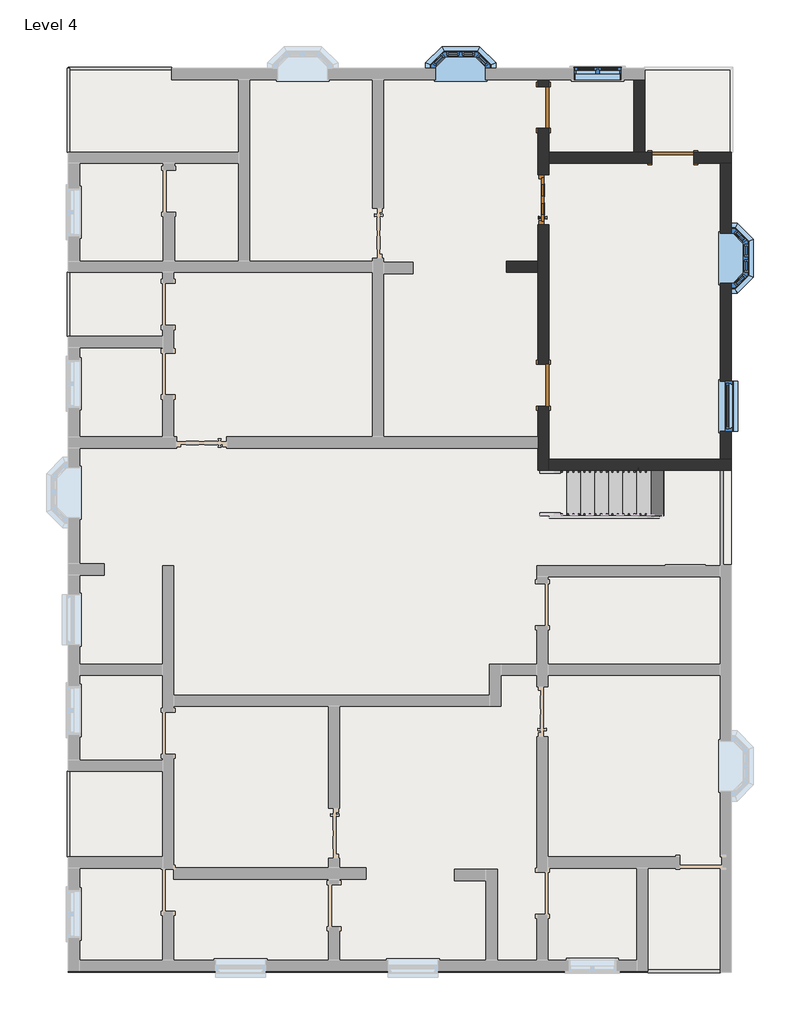
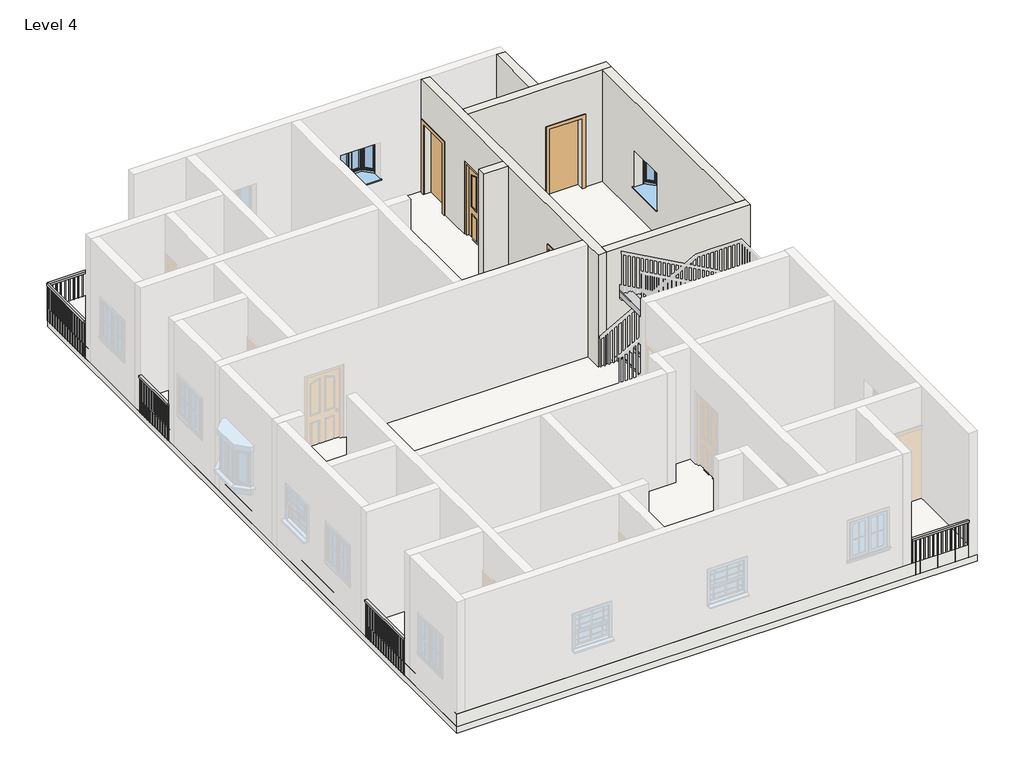
# One storey, part 2 of 4: 6 walls, 5 railings, 4 doors, 4 windows, 1 roof, 1 slab, 1 stair flight.
"""IFC4 building model written with IfcOpenShell, lengths in millimetres."""

from ifc_helpers import new_model, si_unit, frame, origin, place, context, project, spatial, polyline, outline, extrude, faceted_brep, transform, mapped, element, save
from components import doors_extsgl_12_910x2110mm_9a09825e, door_53b1b562, stair_flight_b1286695, window_910x910mm_67ef725a, window_c29befe5, windows_sash_w_bars_1_910x910mm_b688f793

model = new_model("IFC4")

# Units and contexts
model_context = context("Model", 3, world=origin())
ifc_project = project(units=[si_unit("LENGTHUNIT", "METRE", prefix="MILLI")], contexts=[model_context])

# Site, building, storey
site = spatial("IfcSite", under=ifc_project)
building = spatial("IfcBuilding", under=site)
storey = spatial("IfcBuildingStorey", under=building, Name="Level 4", Elevation=9144.0)

# Doors
placement = place(None, origin())
doors_extsgl_12_910x2110mm_shape = doors_extsgl_12_910x2110mm_9a09825e(model_context)
element("IfcDoor", 1, ObjectType="Doors_ExtSgl_12 : 910x2110mm", at=placement, inside=storey, context=model_context, shape_type="MappedRepresentation", body=[
    mapped(doors_extsgl_12_910x2110mm_shape, transform((1600.6941283, 5934.0547293, 9144.0), x_axis=(0.0, 1.0, 0.0), y_axis=(-1.0, 0.0, 0.0), z_axis=(0.0, 0.0, 1.0))),
])
door_shape = door_53b1b562(model_context)
element("IfcDoor", 2, ObjectType="Single-Flush : 30\" x 80\"", at=placement, inside=storey, context=model_context, shape_type="MappedRepresentation", body=[
    mapped(door_shape, transform((1600.6941283, 2555.8547293, 9144.0), x_axis=(0.0, 1.0, 0.0), y_axis=(-1.0, 0.0, 0.0), z_axis=(0.0, 0.0, 1.0))),
])
element("IfcDoor", 3, ObjectType="Single-Flush : 30\" x 80\"", at=placement, inside=storey, context=model_context, shape_type="MappedRepresentation", body=[
    mapped(door_shape, transform((1600.6941283, 7610.4547293, 9144.0), x_axis=(0.0, 1.0, 0.0), y_axis=(-1.0, 0.0, 0.0), z_axis=(0.0, 0.0, 1.0))),
])
element("IfcDoor", 4, ObjectType="Single-Flush : 30\" x 80\"", at=placement, inside=storey, context=model_context, shape_type="MappedRepresentation", body=[
    mapped(door_shape, transform((3962.8941283, 6696.0547293, 9144.0), x_axis=(-1.0, 0.0, 0.0), y_axis=(0.0, -1.0, 0.0), z_axis=(0.0, 0.0, 1.0))),
])

# Railings
element("IfcRailing", 5, ObjectType="Handrail - Rectangular", at=placement, inside=storey, context=model_context, shape_type="SweptSolid", body=[
    extrude(outline(polyline([(-7073.4058717, 4609.0339901), (-7022.6058717, 4609.0339901), (-7022.6058717, 3444.8547293), (-7073.4058717, 3444.8547293), (-7073.4058717, 4609.0339901)])), frame((0.0, 0.0, 10007.6), z_axis=(0.0, 0.0, 1.0), x_axis=(1.0, 0.0, 0.0)), (0.0, 0.0, 1.0), 50.8),
    extrude(outline(polyline([(-7057.5308717, 3500.9589901), (-7038.4808717, 3500.9589901), (-7038.4808717, 3481.9089901), (-7057.5308717, 3481.9089901), (-7057.5308717, 3500.9589901)])), frame((0.0, 0.0, 9144.0), z_axis=(0.0, 0.0, 1.0), x_axis=(1.0, 0.0, 0.0)), (0.0, 0.0, 1.0), 863.6),
    extrude(outline(polyline([(-7057.5308717, 3602.5589901), (-7038.4808717, 3602.5589901), (-7038.4808717, 3583.5089901), (-7057.5308717, 3583.5089901), (-7057.5308717, 3602.5589901)])), frame((0.0, 0.0, 9144.0), z_axis=(0.0, 0.0, 1.0), x_axis=(1.0, 0.0, 0.0)), (0.0, 0.0, 1.0), 863.6),
    extrude(outline(polyline([(-7057.5308717, 3704.1589901), (-7038.4808717, 3704.1589901), (-7038.4808717, 3685.1089901), (-7057.5308717, 3685.1089901), (-7057.5308717, 3704.1589901)])), frame((0.0, 0.0, 9144.0), z_axis=(0.0, 0.0, 1.0), x_axis=(1.0, 0.0, 0.0)), (0.0, 0.0, 1.0), 863.6),
    extrude(outline(polyline([(-7057.5308717, 3805.7589901), (-7038.4808717, 3805.7589901), (-7038.4808717, 3786.7089901), (-7057.5308717, 3786.7089901), (-7057.5308717, 3805.7589901)])), frame((0.0, 0.0, 9144.0), z_axis=(0.0, 0.0, 1.0), x_axis=(1.0, 0.0, 0.0)), (0.0, 0.0, 1.0), 863.6),
    extrude(outline(polyline([(-7057.5308717, 3907.3589901), (-7038.4808717, 3907.3589901), (-7038.4808717, 3888.3089901), (-7057.5308717, 3888.3089901), (-7057.5308717, 3907.3589901)])), frame((0.0, 0.0, 9144.0), z_axis=(0.0, 0.0, 1.0), x_axis=(1.0, 0.0, 0.0)), (0.0, 0.0, 1.0), 863.6),
    extrude(outline(polyline([(-7057.5308717, 4008.9589901), (-7038.4808717, 4008.9589901), (-7038.4808717, 3989.9089901), (-7057.5308717, 3989.9089901), (-7057.5308717, 4008.9589901)])), frame((0.0, 0.0, 9144.0), z_axis=(0.0, 0.0, 1.0), x_axis=(1.0, 0.0, 0.0)), (0.0, 0.0, 1.0), 863.6),
    extrude(outline(polyline([(-7057.5308717, 4110.5589901), (-7038.4808717, 4110.5589901), (-7038.4808717, 4091.5089901), (-7057.5308717, 4091.5089901), (-7057.5308717, 4110.5589901)])), frame((0.0, 0.0, 9144.0), z_axis=(0.0, 0.0, 1.0), x_axis=(1.0, 0.0, 0.0)), (0.0, 0.0, 1.0), 863.6),
    extrude(outline(polyline([(-7057.5308717, 4212.1589901), (-7038.4808717, 4212.1589901), (-7038.4808717, 4193.1089901), (-7057.5308717, 4193.1089901), (-7057.5308717, 4212.1589901)])), frame((0.0, 0.0, 9144.0), z_axis=(0.0, 0.0, 1.0), x_axis=(1.0, 0.0, 0.0)), (0.0, 0.0, 1.0), 863.6),
    extrude(outline(polyline([(-7057.5308717, 4313.7589901), (-7038.4808717, 4313.7589901), (-7038.4808717, 4294.7089901), (-7057.5308717, 4294.7089901), (-7057.5308717, 4313.7589901)])), frame((0.0, 0.0, 9144.0), z_axis=(0.0, 0.0, 1.0), x_axis=(1.0, 0.0, 0.0)), (0.0, 0.0, 1.0), 863.6),
    extrude(outline(polyline([(-7057.5308717, 4415.3589901), (-7038.4808717, 4415.3589901), (-7038.4808717, 4396.3089901), (-7057.5308717, 4396.3089901), (-7057.5308717, 4415.3589901)])), frame((0.0, 0.0, 9144.0), z_axis=(0.0, 0.0, 1.0), x_axis=(1.0, 0.0, 0.0)), (0.0, 0.0, 1.0), 863.6),
    extrude(outline(polyline([(-7057.5308717, 4516.9589901), (-7038.4808717, 4516.9589901), (-7038.4808717, 4497.9089901), (-7057.5308717, 4497.9089901), (-7057.5308717, 4516.9589901)])), frame((0.0, 0.0, 9144.0), z_axis=(0.0, 0.0, 1.0), x_axis=(1.0, 0.0, 0.0)), (0.0, 0.0, 1.0), 863.6),
    extrude(outline(polyline([(-7057.5308717, 3463.9047293), (-7038.4808717, 3463.9047293), (-7038.4808717, 3444.8547293), (-7057.5308717, 3444.8547293), (-7057.5308717, 3463.9047293)])), frame((0.0, 0.0, 9144.0), z_axis=(0.0, 0.0, 1.0), x_axis=(1.0, 0.0, 0.0)), (0.0, 0.0, 1.0), 863.6),
    extrude(outline(polyline([(-7057.5308717, 4609.0339901), (-7038.4808717, 4609.0339901), (-7038.4808717, 4589.9839901), (-7057.5308717, 4589.9839901), (-7057.5308717, 4609.0339901)])), frame((0.0, 0.0, 9144.0), z_axis=(0.0, 0.0, 1.0), x_axis=(1.0, 0.0, 0.0)), (0.0, 0.0, 1.0), 863.6),
])
element("IfcRailing", 6, ObjectType="Handrail - Rectangular", at=placement, inside=storey, context=model_context, shape_type="SweptSolid", body=[
    extrude(outline(polyline([(-7073.4058717, -4474.6886333), (-7022.6058717, -4474.6886333), (-7022.6058717, -6029.3452707), (-7073.4058717, -6029.3452707), (-7073.4058717, -4474.6886333)])), frame((0.0, 0.0, 10007.6), z_axis=(0.0, 0.0, 1.0), x_axis=(1.0, 0.0, 0.0)), (0.0, 0.0, 1.0), 50.8),
    extrude(outline(polyline([(-7057.5308717, -5989.1636333), (-7038.4808717, -5989.1636333), (-7038.4808717, -6008.2136333), (-7057.5308717, -6008.2136333), (-7057.5308717, -5989.1636333)])), frame((0.0, 0.0, 9144.0), z_axis=(0.0, 0.0, 1.0), x_axis=(1.0, 0.0, 0.0)), (0.0, 0.0, 1.0), 863.6),
    extrude(outline(polyline([(-7057.5308717, -5887.5636333), (-7038.4808717, -5887.5636333), (-7038.4808717, -5906.6136333), (-7057.5308717, -5906.6136333), (-7057.5308717, -5887.5636333)])), frame((0.0, 0.0, 9144.0), z_axis=(0.0, 0.0, 1.0), x_axis=(1.0, 0.0, 0.0)), (0.0, 0.0, 1.0), 863.6),
    extrude(outline(polyline([(-7057.5308717, -5785.9636333), (-7038.4808717, -5785.9636333), (-7038.4808717, -5805.0136333), (-7057.5308717, -5805.0136333), (-7057.5308717, -5785.9636333)])), frame((0.0, 0.0, 9144.0), z_axis=(0.0, 0.0, 1.0), x_axis=(1.0, 0.0, 0.0)), (0.0, 0.0, 1.0), 863.6),
    extrude(outline(polyline([(-7057.5308717, -5684.3636333), (-7038.4808717, -5684.3636333), (-7038.4808717, -5703.4136333), (-7057.5308717, -5703.4136333), (-7057.5308717, -5684.3636333)])), frame((0.0, 0.0, 9144.0), z_axis=(0.0, 0.0, 1.0), x_axis=(1.0, 0.0, 0.0)), (0.0, 0.0, 1.0), 863.6),
    extrude(outline(polyline([(-7057.5308717, -5582.7636333), (-7038.4808717, -5582.7636333), (-7038.4808717, -5601.8136333), (-7057.5308717, -5601.8136333), (-7057.5308717, -5582.7636333)])), frame((0.0, 0.0, 9144.0), z_axis=(0.0, 0.0, 1.0), x_axis=(1.0, 0.0, 0.0)), (0.0, 0.0, 1.0), 863.6),
    extrude(outline(polyline([(-7057.5308717, -5481.1636333), (-7038.4808717, -5481.1636333), (-7038.4808717, -5500.2136333), (-7057.5308717, -5500.2136333), (-7057.5308717, -5481.1636333)])), frame((0.0, 0.0, 9144.0), z_axis=(0.0, 0.0, 1.0), x_axis=(1.0, 0.0, 0.0)), (0.0, 0.0, 1.0), 863.6),
    extrude(outline(polyline([(-7057.5308717, -5379.5636333), (-7038.4808717, -5379.5636333), (-7038.4808717, -5398.6136333), (-7057.5308717, -5398.6136333), (-7057.5308717, -5379.5636333)])), frame((0.0, 0.0, 9144.0), z_axis=(0.0, 0.0, 1.0), x_axis=(1.0, 0.0, 0.0)), (0.0, 0.0, 1.0), 863.6),
    extrude(outline(polyline([(-7057.5308717, -5277.9636333), (-7038.4808717, -5277.9636333), (-7038.4808717, -5297.0136333), (-7057.5308717, -5297.0136333), (-7057.5308717, -5277.9636333)])), frame((0.0, 0.0, 9144.0), z_axis=(0.0, 0.0, 1.0), x_axis=(1.0, 0.0, 0.0)), (0.0, 0.0, 1.0), 863.6),
    extrude(outline(polyline([(-7057.5308717, -5176.3636333), (-7038.4808717, -5176.3636333), (-7038.4808717, -5195.4136333), (-7057.5308717, -5195.4136333), (-7057.5308717, -5176.3636333)])), frame((0.0, 0.0, 9144.0), z_axis=(0.0, 0.0, 1.0), x_axis=(1.0, 0.0, 0.0)), (0.0, 0.0, 1.0), 863.6),
    extrude(outline(polyline([(-7057.5308717, -5074.7636333), (-7038.4808717, -5074.7636333), (-7038.4808717, -5093.8136333), (-7057.5308717, -5093.8136333), (-7057.5308717, -5074.7636333)])), frame((0.0, 0.0, 9144.0), z_axis=(0.0, 0.0, 1.0), x_axis=(1.0, 0.0, 0.0)), (0.0, 0.0, 1.0), 863.6),
    extrude(outline(polyline([(-7057.5308717, -4973.1636333), (-7038.4808717, -4973.1636333), (-7038.4808717, -4992.2136333), (-7057.5308717, -4992.2136333), (-7057.5308717, -4973.1636333)])), frame((0.0, 0.0, 9144.0), z_axis=(0.0, 0.0, 1.0), x_axis=(1.0, 0.0, 0.0)), (0.0, 0.0, 1.0), 863.6),
    extrude(outline(polyline([(-7057.5308717, -4871.5636333), (-7038.4808717, -4871.5636333), (-7038.4808717, -4890.6136333), (-7057.5308717, -4890.6136333), (-7057.5308717, -4871.5636333)])), frame((0.0, 0.0, 9144.0), z_axis=(0.0, 0.0, 1.0), x_axis=(1.0, 0.0, 0.0)), (0.0, 0.0, 1.0), 863.6),
    extrude(outline(polyline([(-7057.5308717, -4769.9636333), (-7038.4808717, -4769.9636333), (-7038.4808717, -4789.0136333), (-7057.5308717, -4789.0136333), (-7057.5308717, -4769.9636333)])), frame((0.0, 0.0, 9144.0), z_axis=(0.0, 0.0, 1.0), x_axis=(1.0, 0.0, 0.0)), (0.0, 0.0, 1.0), 863.6),
    extrude(outline(polyline([(-7057.5308717, -4668.3636333), (-7038.4808717, -4668.3636333), (-7038.4808717, -4687.4136333), (-7057.5308717, -4687.4136333), (-7057.5308717, -4668.3636333)])), frame((0.0, 0.0, 9144.0), z_axis=(0.0, 0.0, 1.0), x_axis=(1.0, 0.0, 0.0)), (0.0, 0.0, 1.0), 863.6),
    extrude(outline(polyline([(-7057.5308717, -4566.7636333), (-7038.4808717, -4566.7636333), (-7038.4808717, -4585.8136333), (-7057.5308717, -4585.8136333), (-7057.5308717, -4566.7636333)])), frame((0.0, 0.0, 9144.0), z_axis=(0.0, 0.0, 1.0), x_axis=(1.0, 0.0, 0.0)), (0.0, 0.0, 1.0), 863.6),
    extrude(outline(polyline([(-7057.5308717, -6010.2952707), (-7038.4808717, -6010.2952707), (-7038.4808717, -6029.3452707), (-7057.5308717, -6029.3452707), (-7057.5308717, -6010.2952707)])), frame((0.0, 0.0, 9144.0), z_axis=(0.0, 0.0, 1.0), x_axis=(1.0, 0.0, 0.0)), (0.0, 0.0, 1.0), 863.6),
    extrude(outline(polyline([(-7057.5308717, -4474.6886333), (-7038.4808717, -4474.6886333), (-7038.4808717, -4493.7386333), (-7057.5308717, -4493.7386333), (-7057.5308717, -4474.6886333)])), frame((0.0, 0.0, 9144.0), z_axis=(0.0, 0.0, 1.0), x_axis=(1.0, 0.0, 0.0)), (0.0, 0.0, 1.0), 863.6),
])
element("IfcRailing", 7, ObjectType="Handrail - Rectangular", at=placement, inside=storey, context=model_context, shape_type="SweptSolid", body=[
    extrude(outline(polyline([(3505.6941283, -8137.5452707), (3505.6941283, -8086.7452707), (4826.4941283, -8086.7452707), (4826.4941283, -8137.5452707), (3505.6941283, -8137.5452707)])), frame((0.0, 0.0, 10007.6), z_axis=(0.0, 0.0, 1.0), x_axis=(1.0, 0.0, 0.0)), (0.0, 0.0, 1.0), 50.8),
    extrude(outline(polyline([(4715.3691283, -8121.6702707), (4715.3691283, -8102.6202707), (4734.4191283, -8102.6202707), (4734.4191283, -8121.6702707), (4715.3691283, -8121.6702707)])), frame((0.0, 0.0, 9144.0), z_axis=(0.0, 0.0, 1.0), x_axis=(1.0, 0.0, 0.0)), (0.0, 0.0, 1.0), 863.6),
    extrude(outline(polyline([(4613.7691283, -8121.6702707), (4613.7691283, -8102.6202707), (4632.8191283, -8102.6202707), (4632.8191283, -8121.6702707), (4613.7691283, -8121.6702707)])), frame((0.0, 0.0, 9144.0), z_axis=(0.0, 0.0, 1.0), x_axis=(1.0, 0.0, 0.0)), (0.0, 0.0, 1.0), 863.6),
    extrude(outline(polyline([(4512.1691283, -8121.6702707), (4512.1691283, -8102.6202707), (4531.2191283, -8102.6202707), (4531.2191283, -8121.6702707), (4512.1691283, -8121.6702707)])), frame((0.0, 0.0, 9144.0), z_axis=(0.0, 0.0, 1.0), x_axis=(1.0, 0.0, 0.0)), (0.0, 0.0, 1.0), 863.6),
    extrude(outline(polyline([(4410.5691283, -8121.6702707), (4410.5691283, -8102.6202707), (4429.6191283, -8102.6202707), (4429.6191283, -8121.6702707), (4410.5691283, -8121.6702707)])), frame((0.0, 0.0, 9144.0), z_axis=(0.0, 0.0, 1.0), x_axis=(1.0, 0.0, 0.0)), (0.0, 0.0, 1.0), 863.6),
    extrude(outline(polyline([(4308.9691283, -8121.6702707), (4308.9691283, -8102.6202707), (4328.0191283, -8102.6202707), (4328.0191283, -8121.6702707), (4308.9691283, -8121.6702707)])), frame((0.0, 0.0, 9144.0), z_axis=(0.0, 0.0, 1.0), x_axis=(1.0, 0.0, 0.0)), (0.0, 0.0, 1.0), 863.6),
    extrude(outline(polyline([(4207.3691283, -8121.6702707), (4207.3691283, -8102.6202707), (4226.4191283, -8102.6202707), (4226.4191283, -8121.6702707), (4207.3691283, -8121.6702707)])), frame((0.0, 0.0, 9144.0), z_axis=(0.0, 0.0, 1.0), x_axis=(1.0, 0.0, 0.0)), (0.0, 0.0, 1.0), 863.6),
    extrude(outline(polyline([(4105.7691283, -8121.6702707), (4105.7691283, -8102.6202707), (4124.8191283, -8102.6202707), (4124.8191283, -8121.6702707), (4105.7691283, -8121.6702707)])), frame((0.0, 0.0, 9144.0), z_axis=(0.0, 0.0, 1.0), x_axis=(1.0, 0.0, 0.0)), (0.0, 0.0, 1.0), 863.6),
    extrude(outline(polyline([(4004.1691283, -8121.6702707), (4004.1691283, -8102.6202707), (4023.2191283, -8102.6202707), (4023.2191283, -8121.6702707), (4004.1691283, -8121.6702707)])), frame((0.0, 0.0, 9144.0), z_axis=(0.0, 0.0, 1.0), x_axis=(1.0, 0.0, 0.0)), (0.0, 0.0, 1.0), 863.6),
    extrude(outline(polyline([(3902.5691283, -8121.6702707), (3902.5691283, -8102.6202707), (3921.6191283, -8102.6202707), (3921.6191283, -8121.6702707), (3902.5691283, -8121.6702707)])), frame((0.0, 0.0, 9144.0), z_axis=(0.0, 0.0, 1.0), x_axis=(1.0, 0.0, 0.0)), (0.0, 0.0, 1.0), 863.6),
    extrude(outline(polyline([(3800.9691283, -8121.6702707), (3800.9691283, -8102.6202707), (3820.0191283, -8102.6202707), (3820.0191283, -8121.6702707), (3800.9691283, -8121.6702707)])), frame((0.0, 0.0, 9144.0), z_axis=(0.0, 0.0, 1.0), x_axis=(1.0, 0.0, 0.0)), (0.0, 0.0, 1.0), 863.6),
    extrude(outline(polyline([(3699.3691283, -8121.6702707), (3699.3691283, -8102.6202707), (3718.4191283, -8102.6202707), (3718.4191283, -8121.6702707), (3699.3691283, -8121.6702707)])), frame((0.0, 0.0, 9144.0), z_axis=(0.0, 0.0, 1.0), x_axis=(1.0, 0.0, 0.0)), (0.0, 0.0, 1.0), 863.6),
    extrude(outline(polyline([(3597.7691283, -8121.6702707), (3597.7691283, -8102.6202707), (3616.8191283, -8102.6202707), (3616.8191283, -8121.6702707), (3597.7691283, -8121.6702707)])), frame((0.0, 0.0, 9144.0), z_axis=(0.0, 0.0, 1.0), x_axis=(1.0, 0.0, 0.0)), (0.0, 0.0, 1.0), 863.6),
    extrude(outline(polyline([(4807.4441283, -8121.6702707), (4807.4441283, -8102.6202707), (4826.4941283, -8102.6202707), (4826.4941283, -8121.6702707), (4807.4441283, -8121.6702707)])), frame((0.0, 0.0, 9144.0), z_axis=(0.0, 0.0, 1.0), x_axis=(1.0, 0.0, 0.0)), (0.0, 0.0, 1.0), 863.6),
    extrude(outline(polyline([(3505.6941283, -8121.6702707), (3505.6941283, -8102.6202707), (3524.7441283, -8102.6202707), (3524.7441283, -8121.6702707), (3505.6941283, -8121.6702707)])), frame((0.0, 0.0, 9144.0), z_axis=(0.0, 0.0, 1.0), x_axis=(1.0, 0.0, 0.0)), (0.0, 0.0, 1.0), 863.6),
])
element("IfcRailing", 8, ObjectType="Handrail - Rectangular", at=placement, inside=storey, context=model_context, shape_type="SweptSolid", body=[
    extrude(outline(polyline([(-7022.6058717, 6797.6547293), (-7073.4058717, 6797.6547293), (-7073.4058717, 8321.6547293), (-7022.6058717, 8321.6547293), (-7022.6058717, 6797.6547293)])), frame((0.0, 0.0, 10007.6), z_axis=(0.0, 0.0, 1.0), x_axis=(1.0, 0.0, 0.0)), (0.0, 0.0, 1.0), 50.8),
    extrude(outline(polyline([(-7038.4808717, 8210.5297293), (-7057.5308717, 8210.5297293), (-7057.5308717, 8229.5797293), (-7038.4808717, 8229.5797293), (-7038.4808717, 8210.5297293)])), frame((0.0, 0.0, 9144.0), z_axis=(0.0, 0.0, 1.0), x_axis=(1.0, 0.0, 0.0)), (0.0, 0.0, 1.0), 863.6),
    extrude(outline(polyline([(-7038.4808717, 8108.9297293), (-7057.5308717, 8108.9297293), (-7057.5308717, 8127.9797293), (-7038.4808717, 8127.9797293), (-7038.4808717, 8108.9297293)])), frame((0.0, 0.0, 9144.0), z_axis=(0.0, 0.0, 1.0), x_axis=(1.0, 0.0, 0.0)), (0.0, 0.0, 1.0), 863.6),
    extrude(outline(polyline([(-7038.4808717, 8007.3297293), (-7057.5308717, 8007.3297293), (-7057.5308717, 8026.3797293), (-7038.4808717, 8026.3797293), (-7038.4808717, 8007.3297293)])), frame((0.0, 0.0, 9144.0), z_axis=(0.0, 0.0, 1.0), x_axis=(1.0, 0.0, 0.0)), (0.0, 0.0, 1.0), 863.6),
    extrude(outline(polyline([(-7038.4808717, 7905.7297293), (-7057.5308717, 7905.7297293), (-7057.5308717, 7924.7797293), (-7038.4808717, 7924.7797293), (-7038.4808717, 7905.7297293)])), frame((0.0, 0.0, 9144.0), z_axis=(0.0, 0.0, 1.0), x_axis=(1.0, 0.0, 0.0)), (0.0, 0.0, 1.0), 863.6),
    extrude(outline(polyline([(-7038.4808717, 7804.1297293), (-7057.5308717, 7804.1297293), (-7057.5308717, 7823.1797293), (-7038.4808717, 7823.1797293), (-7038.4808717, 7804.1297293)])), frame((0.0, 0.0, 9144.0), z_axis=(0.0, 0.0, 1.0), x_axis=(1.0, 0.0, 0.0)), (0.0, 0.0, 1.0), 863.6),
    extrude(outline(polyline([(-7038.4808717, 7702.5297293), (-7057.5308717, 7702.5297293), (-7057.5308717, 7721.5797293), (-7038.4808717, 7721.5797293), (-7038.4808717, 7702.5297293)])), frame((0.0, 0.0, 9144.0), z_axis=(0.0, 0.0, 1.0), x_axis=(1.0, 0.0, 0.0)), (0.0, 0.0, 1.0), 863.6),
    extrude(outline(polyline([(-7038.4808717, 7600.9297293), (-7057.5308717, 7600.9297293), (-7057.5308717, 7619.9797293), (-7038.4808717, 7619.9797293), (-7038.4808717, 7600.9297293)])), frame((0.0, 0.0, 9144.0), z_axis=(0.0, 0.0, 1.0), x_axis=(1.0, 0.0, 0.0)), (0.0, 0.0, 1.0), 863.6),
    extrude(outline(polyline([(-7038.4808717, 7499.3297293), (-7057.5308717, 7499.3297293), (-7057.5308717, 7518.3797293), (-7038.4808717, 7518.3797293), (-7038.4808717, 7499.3297293)])), frame((0.0, 0.0, 9144.0), z_axis=(0.0, 0.0, 1.0), x_axis=(1.0, 0.0, 0.0)), (0.0, 0.0, 1.0), 863.6),
    extrude(outline(polyline([(-7038.4808717, 7397.7297293), (-7057.5308717, 7397.7297293), (-7057.5308717, 7416.7797293), (-7038.4808717, 7416.7797293), (-7038.4808717, 7397.7297293)])), frame((0.0, 0.0, 9144.0), z_axis=(0.0, 0.0, 1.0), x_axis=(1.0, 0.0, 0.0)), (0.0, 0.0, 1.0), 863.6),
    extrude(outline(polyline([(-7038.4808717, 7296.1297293), (-7057.5308717, 7296.1297293), (-7057.5308717, 7315.1797293), (-7038.4808717, 7315.1797293), (-7038.4808717, 7296.1297293)])), frame((0.0, 0.0, 9144.0), z_axis=(0.0, 0.0, 1.0), x_axis=(1.0, 0.0, 0.0)), (0.0, 0.0, 1.0), 863.6),
    extrude(outline(polyline([(-7038.4808717, 7194.5297293), (-7057.5308717, 7194.5297293), (-7057.5308717, 7213.5797293), (-7038.4808717, 7213.5797293), (-7038.4808717, 7194.5297293)])), frame((0.0, 0.0, 9144.0), z_axis=(0.0, 0.0, 1.0), x_axis=(1.0, 0.0, 0.0)), (0.0, 0.0, 1.0), 863.6),
    extrude(outline(polyline([(-7038.4808717, 7092.9297293), (-7057.5308717, 7092.9297293), (-7057.5308717, 7111.9797293), (-7038.4808717, 7111.9797293), (-7038.4808717, 7092.9297293)])), frame((0.0, 0.0, 9144.0), z_axis=(0.0, 0.0, 1.0), x_axis=(1.0, 0.0, 0.0)), (0.0, 0.0, 1.0), 863.6),
    extrude(outline(polyline([(-7038.4808717, 6991.3297293), (-7057.5308717, 6991.3297293), (-7057.5308717, 7010.3797293), (-7038.4808717, 7010.3797293), (-7038.4808717, 6991.3297293)])), frame((0.0, 0.0, 9144.0), z_axis=(0.0, 0.0, 1.0), x_axis=(1.0, 0.0, 0.0)), (0.0, 0.0, 1.0), 863.6),
    extrude(outline(polyline([(-7038.4808717, 6889.7297293), (-7057.5308717, 6889.7297293), (-7057.5308717, 6908.7797293), (-7038.4808717, 6908.7797293), (-7038.4808717, 6889.7297293)])), frame((0.0, 0.0, 9144.0), z_axis=(0.0, 0.0, 1.0), x_axis=(1.0, 0.0, 0.0)), (0.0, 0.0, 1.0), 863.6),
    extrude(outline(polyline([(-7038.4808717, 8302.6047293), (-7057.5308717, 8302.6047293), (-7057.5308717, 8321.6547293), (-7038.4808717, 8321.6547293), (-7038.4808717, 8302.6047293)])), frame((0.0, 0.0, 9144.0), z_axis=(0.0, 0.0, 1.0), x_axis=(1.0, 0.0, 0.0)), (0.0, 0.0, 1.0), 863.6),
    extrude(outline(polyline([(-7038.4808717, 6797.6547293), (-7057.5308717, 6797.6547293), (-7057.5308717, 6816.7047293), (-7038.4808717, 6816.7047293), (-7038.4808717, 6797.6547293)])), frame((0.0, 0.0, 9144.0), z_axis=(0.0, 0.0, 1.0), x_axis=(1.0, 0.0, 0.0)), (0.0, 0.0, 1.0), 863.6),
])
element("IfcRailing", 9, ObjectType="Handrail - Rectangular", at=placement, inside=storey, context=model_context, shape_type="SweptSolid", body=[
    extrude(outline(polyline([(-7048.0058717, 8296.2547293), (-7048.0058717, 8347.0547293), (-5168.4058717, 8347.0547293), (-5168.4058717, 8296.2547293), (-7048.0058717, 8296.2547293)])), frame((0.0, 0.0, 10007.6), z_axis=(0.0, 0.0, 1.0), x_axis=(1.0, 0.0, 0.0)), (0.0, 0.0, 1.0), 50.8),
    extrude(outline(polyline([(-5228.7308717, 8312.1297293), (-5228.7308717, 8331.1797293), (-5209.6808717, 8331.1797293), (-5209.6808717, 8312.1297293), (-5228.7308717, 8312.1297293)])), frame((0.0, 0.0, 9144.0), z_axis=(0.0, 0.0, 1.0), x_axis=(1.0, 0.0, 0.0)), (0.0, 0.0, 1.0), 863.6),
    extrude(outline(polyline([(-5330.3308717, 8312.1297293), (-5330.3308717, 8331.1797293), (-5311.2808717, 8331.1797293), (-5311.2808717, 8312.1297293), (-5330.3308717, 8312.1297293)])), frame((0.0, 0.0, 9144.0), z_axis=(0.0, 0.0, 1.0), x_axis=(1.0, 0.0, 0.0)), (0.0, 0.0, 1.0), 863.6),
    extrude(outline(polyline([(-5431.9308717, 8312.1297293), (-5431.9308717, 8331.1797293), (-5412.8808717, 8331.1797293), (-5412.8808717, 8312.1297293), (-5431.9308717, 8312.1297293)])), frame((0.0, 0.0, 9144.0), z_axis=(0.0, 0.0, 1.0), x_axis=(1.0, 0.0, 0.0)), (0.0, 0.0, 1.0), 863.6),
    extrude(outline(polyline([(-5533.5308717, 8312.1297293), (-5533.5308717, 8331.1797293), (-5514.4808717, 8331.1797293), (-5514.4808717, 8312.1297293), (-5533.5308717, 8312.1297293)])), frame((0.0, 0.0, 9144.0), z_axis=(0.0, 0.0, 1.0), x_axis=(1.0, 0.0, 0.0)), (0.0, 0.0, 1.0), 863.6),
    extrude(outline(polyline([(-5635.1308717, 8312.1297293), (-5635.1308717, 8331.1797293), (-5616.0808717, 8331.1797293), (-5616.0808717, 8312.1297293), (-5635.1308717, 8312.1297293)])), frame((0.0, 0.0, 9144.0), z_axis=(0.0, 0.0, 1.0), x_axis=(1.0, 0.0, 0.0)), (0.0, 0.0, 1.0), 863.6),
    extrude(outline(polyline([(-5736.7308717, 8312.1297293), (-5736.7308717, 8331.1797293), (-5717.6808717, 8331.1797293), (-5717.6808717, 8312.1297293), (-5736.7308717, 8312.1297293)])), frame((0.0, 0.0, 9144.0), z_axis=(0.0, 0.0, 1.0), x_axis=(1.0, 0.0, 0.0)), (0.0, 0.0, 1.0), 863.6),
    extrude(outline(polyline([(-5838.3308717, 8312.1297293), (-5838.3308717, 8331.1797293), (-5819.2808717, 8331.1797293), (-5819.2808717, 8312.1297293), (-5838.3308717, 8312.1297293)])), frame((0.0, 0.0, 9144.0), z_axis=(0.0, 0.0, 1.0), x_axis=(1.0, 0.0, 0.0)), (0.0, 0.0, 1.0), 863.6),
    extrude(outline(polyline([(-5939.9308717, 8312.1297293), (-5939.9308717, 8331.1797293), (-5920.8808717, 8331.1797293), (-5920.8808717, 8312.1297293), (-5939.9308717, 8312.1297293)])), frame((0.0, 0.0, 9144.0), z_axis=(0.0, 0.0, 1.0), x_axis=(1.0, 0.0, 0.0)), (0.0, 0.0, 1.0), 863.6),
    extrude(outline(polyline([(-6041.5308717, 8312.1297293), (-6041.5308717, 8331.1797293), (-6022.4808717, 8331.1797293), (-6022.4808717, 8312.1297293), (-6041.5308717, 8312.1297293)])), frame((0.0, 0.0, 9144.0), z_axis=(0.0, 0.0, 1.0), x_axis=(1.0, 0.0, 0.0)), (0.0, 0.0, 1.0), 863.6),
    extrude(outline(polyline([(-6143.1308717, 8312.1297293), (-6143.1308717, 8331.1797293), (-6124.0808717, 8331.1797293), (-6124.0808717, 8312.1297293), (-6143.1308717, 8312.1297293)])), frame((0.0, 0.0, 9144.0), z_axis=(0.0, 0.0, 1.0), x_axis=(1.0, 0.0, 0.0)), (0.0, 0.0, 1.0), 863.6),
    extrude(outline(polyline([(-6244.7308717, 8312.1297293), (-6244.7308717, 8331.1797293), (-6225.6808717, 8331.1797293), (-6225.6808717, 8312.1297293), (-6244.7308717, 8312.1297293)])), frame((0.0, 0.0, 9144.0), z_axis=(0.0, 0.0, 1.0), x_axis=(1.0, 0.0, 0.0)), (0.0, 0.0, 1.0), 863.6),
    extrude(outline(polyline([(-6346.3308717, 8312.1297293), (-6346.3308717, 8331.1797293), (-6327.2808717, 8331.1797293), (-6327.2808717, 8312.1297293), (-6346.3308717, 8312.1297293)])), frame((0.0, 0.0, 9144.0), z_axis=(0.0, 0.0, 1.0), x_axis=(1.0, 0.0, 0.0)), (0.0, 0.0, 1.0), 863.6),
    extrude(outline(polyline([(-6447.9308717, 8312.1297293), (-6447.9308717, 8331.1797293), (-6428.8808717, 8331.1797293), (-6428.8808717, 8312.1297293), (-6447.9308717, 8312.1297293)])), frame((0.0, 0.0, 9144.0), z_axis=(0.0, 0.0, 1.0), x_axis=(1.0, 0.0, 0.0)), (0.0, 0.0, 1.0), 863.6),
    extrude(outline(polyline([(-6549.5308717, 8312.1297293), (-6549.5308717, 8331.1797293), (-6530.4808717, 8331.1797293), (-6530.4808717, 8312.1297293), (-6549.5308717, 8312.1297293)])), frame((0.0, 0.0, 9144.0), z_axis=(0.0, 0.0, 1.0), x_axis=(1.0, 0.0, 0.0)), (0.0, 0.0, 1.0), 863.6),
    extrude(outline(polyline([(-6651.1308717, 8312.1297293), (-6651.1308717, 8331.1797293), (-6632.0808717, 8331.1797293), (-6632.0808717, 8312.1297293), (-6651.1308717, 8312.1297293)])), frame((0.0, 0.0, 9144.0), z_axis=(0.0, 0.0, 1.0), x_axis=(1.0, 0.0, 0.0)), (0.0, 0.0, 1.0), 863.6),
    extrude(outline(polyline([(-6752.7308717, 8312.1297293), (-6752.7308717, 8331.1797293), (-6733.6808717, 8331.1797293), (-6733.6808717, 8312.1297293), (-6752.7308717, 8312.1297293)])), frame((0.0, 0.0, 9144.0), z_axis=(0.0, 0.0, 1.0), x_axis=(1.0, 0.0, 0.0)), (0.0, 0.0, 1.0), 863.6),
    extrude(outline(polyline([(-6854.3308717, 8312.1297293), (-6854.3308717, 8331.1797293), (-6835.2808717, 8331.1797293), (-6835.2808717, 8312.1297293), (-6854.3308717, 8312.1297293)])), frame((0.0, 0.0, 9144.0), z_axis=(0.0, 0.0, 1.0), x_axis=(1.0, 0.0, 0.0)), (0.0, 0.0, 1.0), 863.6),
    extrude(outline(polyline([(-6955.9308717, 8312.1297293), (-6955.9308717, 8331.1797293), (-6936.8808717, 8331.1797293), (-6936.8808717, 8312.1297293), (-6955.9308717, 8312.1297293)])), frame((0.0, 0.0, 9144.0), z_axis=(0.0, 0.0, 1.0), x_axis=(1.0, 0.0, 0.0)), (0.0, 0.0, 1.0), 863.6),
    extrude(outline(polyline([(-5187.4558717, 8312.1297293), (-5187.4558717, 8331.1797293), (-5168.4058717, 8331.1797293), (-5168.4058717, 8312.1297293), (-5187.4558717, 8312.1297293)])), frame((0.0, 0.0, 9144.0), z_axis=(0.0, 0.0, 1.0), x_axis=(1.0, 0.0, 0.0)), (0.0, 0.0, 1.0), 863.6),
    extrude(outline(polyline([(-7048.0058717, 8312.1297293), (-7048.0058717, 8331.1797293), (-7028.9558717, 8331.1797293), (-7028.9558717, 8312.1297293), (-7048.0058717, 8312.1297293)])), frame((0.0, 0.0, 9144.0), z_axis=(0.0, 0.0, 1.0), x_axis=(1.0, 0.0, 0.0)), (0.0, 0.0, 1.0), 863.6),
])

# Roof
element("IfcRoof", 10, ObjectType="Generic - 12\"", at=placement, inside=storey, context=model_context, shape_type="SweptSolid", body=[
    extrude(outline(polyline([(-7048.0058717, 8321.6547293), (5029.6941283, 8321.6547293), (5029.6941283, -8124.8452707), (-7048.0058717, -8124.8452707), (-7048.0058717, 8321.6547293)])), frame((0.0, 0.0, 9144.0), z_axis=(0.0, 0.0, 1.0), x_axis=(1.0, 0.0, 0.0)), (0.0, 0.0, 1.0), 304.8),
])

# Slab
element("IfcSlab", 11, ObjectType="Generic - 12\"", at=placement, inside=storey, context=model_context, shape_type="SweptSolid", body=[
    extrude(outline(polyline([(5029.6941283, 8321.6547293), (5029.6941283, -8124.8452707), (-7048.0058717, -8124.8452707), (-7048.0058717, 8321.6547293), (5029.6941283, 8321.6547293)])), frame((0.0, 0.0, 8991.6), z_axis=(0.0, 0.0, 1.0), x_axis=(1.0, 0.0, 0.0)), (0.0, 0.0, 1.0), 152.4),
])

# Stair flight
stair_flight_shape = stair_flight_b1286695(model_context)
element("IfcStairFlight", 12, ObjectType="2\" Tread 1\" Nosing 1/4\" Riser", at=placement, inside=storey, context=model_context, shape_type="MappedRepresentation", body=[
    mapped(stair_flight_shape, transform((0.0, 0.0, 0.0), x_axis=(1.0, 0.0, 0.0), y_axis=(0.0, 1.0, 0.0), z_axis=(0.0, 0.0, 1.0))),
])

# Walls
element("IfcWall", 13, ObjectType="Generic - 4.5\"", at=placement, inside=storey, context=model_context, shape_type="Brep", body=[
    faceted_brep([(1499.0941283, 8118.4547293, 9144.0), (1499.0941283, 7991.4547293, 9144.0), (1499.0941283, 7991.4547293, 11176.0), (1499.0941283, 7229.4547293, 11176.0), (1499.0941283, 7229.4547293, 9144.0), (1499.0941283, 6389.0547293, 9144.0), (1499.0941283, 6389.0547293, 11254.0), (1499.0941283, 5479.0547293, 11254.0), (1499.0941283, 5479.0547293, 9144.0), (1499.0941283, 4812.2339901, 9144.0), (1499.0941283, 4609.0339901, 9144.0), (1499.0941283, 2936.8547293, 9144.0), (1499.0941283, 2936.8547293, 11176.0), (1499.0941283, 2174.8547293, 11176.0), (1499.0941283, 2174.8547293, 9144.0), (1499.0941283, 1616.0547293, 9144.0), (1499.0941283, 1412.8547293, 9144.0), (1499.0941283, 1006.4547293, 9144.0), (1499.0941283, 1006.4547293, 12192.0), (1499.0941283, 1412.8547293, 12192.0), (1499.0941283, 1616.0547293, 12192.0), (1499.0941283, 4609.0339901, 12192.0), (1499.0941283, 4812.2339901, 12192.0), (1499.0941283, 8118.4547293, 12192.0), (1702.2941283, 7991.4547293, 11176.0), (1702.2941283, 7991.4547293, 9144.0), (1702.2941283, 8118.4547293, 9144.0), (1702.2941283, 8118.4547293, 12192.0), (1702.2941283, 6797.6547293, 12192.0), (1702.2941283, 6594.4547293, 12192.0), (1702.2941283, 1209.6547293, 12192.0), (1702.2941283, 1006.4547293, 12192.0), (1702.2941283, 1006.4547293, 9144.0), (1702.2941283, 1209.6547293, 9144.0), (1702.2941283, 2174.8547293, 9144.0), (1702.2941283, 2174.8547293, 11176.0), (1702.2941283, 2936.8547293, 11176.0), (1702.2941283, 2936.8547293, 9144.0), (1702.2941283, 5479.0547293, 9144.0), (1702.2941283, 5479.0547293, 11254.0), (1702.2941283, 6389.0547293, 11254.0), (1702.2941283, 6389.0547293, 9144.0), (1702.2941283, 6594.4547293, 9144.0), (1702.2941283, 6797.6547293, 9144.0), (1702.2941283, 7229.4547293, 9144.0), (1702.2941283, 7229.4547293, 11176.0)], [[[0, 1, 2, 3, 4, 5, 6, 7, 8, 9, 10, 11, 12, 13, 14, 15, 16, 17, 18, 19, 20, 21, 22, 23]], [[24, 25, 26, 27, 28, 29, 30, 31, 32, 33, 34, 35, 36, 37, 38, 39, 40, 41, 42, 43, 44, 45]], [[38, 37, 11, 10, 9, 8]], [[34, 33, 32, 17, 16, 15, 14]], [[26, 25, 1, 0]], [[44, 43, 42, 41, 5, 4]], [[23, 22, 21, 20, 19, 18, 31, 30, 29, 28, 27]], [[0, 23, 27, 26]], [[18, 17, 32, 31]], [[8, 7, 39, 38]], [[6, 5, 41, 40]], [[7, 6, 40, 39]], [[12, 11, 37, 36]], [[13, 12, 36, 35]], [[14, 13, 35, 34]], [[2, 1, 25, 24]], [[3, 2, 24, 45]], [[4, 3, 45, 44]]]),
])
element("IfcWall", 14, ObjectType="Generic - 4.5\"", at=placement, inside=storey, context=model_context, shape_type="Brep", body=[
    faceted_brep([(1702.2941283, 6594.4547293, 9144.0), (3581.8941283, 6594.4547293, 9144.0), (3581.8941283, 6594.4547293, 11176.0), (4343.8941283, 6594.4547293, 11176.0), (4343.8941283, 6594.4547293, 9144.0), (4826.4941283, 6594.4547293, 9144.0), (5029.6941283, 6594.4547293, 9144.0), (5029.6941283, 6594.4547293, 12192.0), (4826.4941283, 6594.4547293, 12192.0), (1702.2941283, 6594.4547293, 12192.0), (3581.8941283, 6797.6547293, 11176.0), (3581.8941283, 6797.6547293, 9144.0), (3454.8941283, 6797.6547293, 9144.0), (3251.6941283, 6797.6547293, 9144.0), (1702.2941283, 6797.6547293, 9144.0), (1702.2941283, 6797.6547293, 12192.0), (3251.6941283, 6797.6547293, 12192.0), (3454.8941283, 6797.6547293, 12192.0), (5029.6941283, 6797.6547293, 12192.0), (5029.6941283, 6797.6547293, 9144.0), (4343.8941283, 6797.6547293, 9144.0), (4343.8941283, 6797.6547293, 11176.0)], [[[0, 1, 2, 3, 4, 5, 6, 7, 8, 9]], [[10, 11, 12, 13, 14, 15, 16, 17, 18, 19, 20, 21]], [[20, 19, 6, 5, 4]], [[14, 13, 12, 11, 1, 0]], [[9, 8, 7, 18, 17, 16, 15]], [[0, 9, 15, 14]], [[2, 1, 11, 10]], [[3, 2, 10, 21]], [[4, 3, 21, 20]], [[7, 6, 19, 18]]]),
])
element("IfcWall", 15, ObjectType="Generic - 4.5\"", at=placement, inside=storey, context=model_context, shape_type="SweptSolid", body=[
    extrude(outline(polyline([(3251.6941283, 6797.6547293), (3251.6941283, 8118.4547293), (3454.8941283, 8118.4547293), (3454.8941283, 6797.6547293), (3251.6941283, 6797.6547293)])), frame((0.0, 0.0, 9144.0), z_axis=(0.0, 0.0, 1.0), x_axis=(1.0, 0.0, 0.0)), (0.0, 0.0, 1.0), 3048.0),
])
element("IfcWall", 16, ObjectType="Generic - 4.5\"", at=placement, inside=storey, context=model_context, shape_type="Brep", body=[
    faceted_brep([(1702.2941283, 1006.4547293, 9144.0), (5029.6941283, 1006.4547293, 9144.0), (5029.6941283, 1006.4547293, 12192.0), (1702.2941283, 1006.4547293, 12192.0), (1702.2941283, 1209.6547293, 9144.0), (1702.2941283, 1209.6547293, 12192.0), (4826.4941283, 1209.6547293, 12192.0), (5029.6941283, 1209.6547293, 12192.0), (5029.6941283, 1209.6547293, 9144.0), (4826.4941283, 1209.6547293, 9144.0)], [[[0, 1, 2, 3]], [[4, 5, 6, 7, 8, 9]], [[1, 0, 4, 9, 8]], [[3, 2, 7, 6, 5]], [[0, 3, 5, 4]], [[2, 1, 8, 7]]]),
])
element("IfcWall", 17, ObjectType="Generic - 4.5\"", at=placement, inside=storey, context=model_context, shape_type="SweptSolid", body=[
    extrude(outline(polyline([(927.5941283, 4812.2339901), (1499.0941283, 4812.2339901), (1499.0941283, 4609.0339901), (927.5941283, 4609.0339901), (927.5941283, 4812.2339901)])), frame((0.0, 0.0, 9144.0), z_axis=(0.0, 0.0, 1.0), x_axis=(1.0, 0.0, 0.0)), (0.0, 0.0, 1.0), 3048.0),
])
element("IfcWall", 18, ObjectType="Generic - 9\"", at=placement, inside=storey, context=model_context, shape_type="SweptSolid", body=[
    extrude(outline(polyline([(6594.4547293, 9144.0), (1209.6547293, 9144.0), (1209.6547293, 12192.0), (6594.4547293, 12192.0), (6594.4547293, 9144.0)]), holes=[polyline([(5322.2547293, 10968.4), (4412.2547293, 10968.4), (4412.2547293, 10058.4), (5322.2547293, 10058.4), (5322.2547293, 10968.4)]), polyline([(2629.8547293, 10058.4), (2629.8547293, 10968.4), (1719.8547293, 10968.4), (1719.8547293, 10058.4), (2629.8547293, 10058.4)])]), frame((4826.4941283, 0.0, 0.0), z_axis=(1.0, 0.0, 0.0), x_axis=(0.0, 1.0, 0.0)), (0.0, 0.0, 1.0), 203.2),
])

# Windows
window_910x910mm_shape = window_910x910mm_67ef725a(model_context)
element("IfcWindow", 19, ObjectType="910x910mm", at=placement, inside=storey, context=model_context, shape_type="MappedRepresentation", body=[
    mapped(window_910x910mm_shape, transform((4919.6375605, 4297.2547293, 8858.4), x_axis=(0.0, -1.0, 0.0), y_axis=(1.0, 0.0, 0.0), z_axis=(0.0, 0.0, 1.0))),
])
element("IfcWindow", 20, ObjectType="910x910mm", at=placement, inside=storey, context=model_context, shape_type="MappedRepresentation", body=[
    mapped(window_910x910mm_shape, transform((665.7441283, 8211.5981615, 8858.4), x_axis=(1.0, 0.0, 0.0), y_axis=(0.0, 1.0, 0.0), z_axis=(0.0, 0.0, 1.0))),
])
window_shape = window_c29befe5(model_context)
element("IfcWindow", 21, ObjectType="Window-Casement-Double : 34\" x 36\"", at=placement, inside=storey, context=model_context, shape_type="MappedRepresentation", body=[
    mapped(window_shape, transform((2591.2941283, 8220.0547293, 9144.0), x_axis=(1.0, 0.0, 0.0), y_axis=(0.0, 1.0, 0.0), z_axis=(0.0, 0.0, 1.0))),
])
windows_sash_w_bars_1_910x910mm_shape = windows_sash_w_bars_1_910x910mm_b688f793(model_context)
element("IfcWindow", 22, ObjectType="Windows_Sash_w-Bars_1 : 910x910mm", at=placement, inside=storey, context=model_context, shape_type="MappedRepresentation", body=[
    mapped(windows_sash_w_bars_1_910x910mm_shape, transform((4928.0941283, 2174.8547293, 9258.4), x_axis=(0.0, -1.0, 0.0), y_axis=(1.0, 0.0, 0.0), z_axis=(0.0, 0.0, 1.0))),
])

save(model, "model.ifc")

# Revit data of these elements
# Type "Doors_ExtSgl_12 : 910x2110mm"
#   Type Mark = "10"
#   Type Comments = "External Single"
#   Operation = "SingleSwingRight"
#   Construction Type Id = "SGL"
#   Keynote = "L20"
#   Analytic Construction = "Large single-glazed windows"
#   Wrap Layers (Int) from Ext = 0' - 6.98819"
#   Wrap Layers (Ext) from Ext = 0' - 4.03543"
#   Visual Light Transmittance = 0.9
#   Thickness = 0' - 1.73228"
#   Stile Top of Lock rail = 3' - 3.37008"
#   Stile Top Rail = 0' - 5.90551"
#   Stile Shutting = 0' - 4.92126"
#   Stile Muntin Rail = 0' - 4.92126"
#   Stile Lock Rail = 0' - 6.88976"
#   Stile Hanging = 0' - 4.92126"
#   Stile Bottom Rail = 0' - 6.88976"
#   Solar Heat Gain Coefficient = 0.86
#   Rough Width = 2' - 11.82677"
#   Rough Height = 6' - 11.07087"
#   O/A Frame Width = 0' - 2.51969"
#   Heat Transfer Coefficient (U) = 0.979472 BTU/(h·ft²·°F)
#   Handle Z Distance = 3' - 3.37008"
#   Glazing Thickness = 0' - 0.94488"
#   FrameWidth = 0' - 1.65354"
#   FrameOffset - External = 0' - 0.98425"
#   FrameDepth = 0' - 3.50394"
#   Door Panel Width = 2' - 7.77165"
#   Door Panel Thickness = 0' - 1.73228"
#   Door Panel Height = 6' - 6.74016"
#   Cill Thickness = 0' - 2.14567"
#   Cill Projection = 0' - 1.1811"
#   Handle X Distance = 0' - 2.95276"
#   Height = 6' - 11.07087"
#   Structural Tolerance = 0' - 0.25591"
#   Tolerance = 0' - 0.11811"
#   Undercut = 0' - 0.15748"
#   Width = 2' - 11.82677"
#   Cill Extension = 0' - 0.98425"
#   Cavity Closer Width = 0' - 1.9685"
#   Cavity Closer Offset from Ext = 0' - 4.03543"
#   Cavity Closer Depth = 0' - 3.34646"
#   Vis - Ironmongery = yes
#   Vis - Cavity Closers = yes
#   Define Thermal Properties by = 1
#   Function = 1
#   Material Glass = Door - Glazing
#   Material Door = Door - Panel
#   Material Frame = Door - Frame/Mullion
#   Material Ironmongery = Door - Handle
#   Wall Closure = (empty or 0)
# Type "Single-Flush : 30\" x 80\""
#   Type Mark = "5"
#   Construction Type Id = "MDOOR"
#   Assembly Code = "C1020"
#   Analytic Construction = "Metal"
#   Thickness = 0' - 2"
#   Heat Transfer Coefficient (U) = 0.651978 BTU/(h·ft²·°F)
#   Height = 6' - 8"
#   Trim Projection Ext = 0' - 1"
#   Trim Projection Int = 0' - 1"
#   Trim Width = 0' - 3"
#   Width = 2' - 6"
#   Define Thermal Properties by = 1
#   Define Thermal Properties by = 1
#   Door Material = Door - Panel
#   Frame Material = Door - Frame
#   Visual Light Transmittance = 0
#   Solar Heat Gain Coefficient = 0
#   Function = (empty or 0)
#   Wall Closure = (empty or 0)
# Type "Handrail - Rectangular"
#   Assembly Code = "C2010400"
#   built-in parameter 1008612 = 0.0416667 (stored number, unit not read)
#   built-in parameter 1008611 = 0.0416667 (stored number, unit not read)
#   built-in parameter 1008609 = 0.333333 (stored number, unit not read)
#   built-in parameter 1008604 = 0.166667 (stored number, unit not read)
#   built-in parameter 1008603 = 0.166667 (stored number, unit not read)
#   Railing Height = 3' - 0"
#   built-in parameter 1008630 = 2
#   built-in parameter 1008610 = 2
#   built-in parameter 1008618 = Baluster - Square : 3/4"
# Type "Generic - 12\""
#   Assembly Code = "B1020"
#   Layers, outside or top first: 1' - 0" no material (function 1)
# Type "Generic - 12\""
#   Assembly Code = "B1010"
#   Function = 0
#   Layers, outside or top first: 0' - 6" no material (function 1)
# Type "Generic - 4.5\""
#   Assembly Code = "B2010"
#   Layers, outside or top first: 0' - 8" no material (function 1)
# Type "Generic - 9\""
#   Assembly Code = "B2010"
#   Layers, outside or top first: 0' - 8" no material (function 1)
# Type "910x910mm"
#   Type Mark = "18"
#   Operation = "UserDefined"
#   Construction Type Id = "GSP4R"
#   Keynote = "L10"
#   Analytic Construction = "1/8 in Pilkington single glazing"
#   Wrap Layers (Ext) from Ext = 0' - 4.03543"
#   Wrap Layers (Int) from Ext = 0' - 6.98819"
#   Window Board Projection = 0' - 0.98425"
#   Window Board Extention = 0' - 0.98425"
#   Visual Light Transmittance = 0.9
#   Solar Heat Gain Coefficient = 0.78
#   Heat Transfer Coefficient (U) = 0.6496 BTU/(h·ft²·°F)
#   Glazing Thickness = 0' - 0.94488"
#   DONT CHANGE - Splay Width = 0' - 7.41997"
#   Rough Width = 2' - 11.82677"
#   Rough Height = 2' - 11.82677"
#   Roof Thickness = 0' - 4.92126"
#   Roof Overhang = 0' - 1.5748"
#   Plinth Thickness = 0' - 6.88976"
#   Height = 2' - 11.82677"
#   Width = 2' - 11.82677"
#   Frame Depth = 0' - 2.55906"
#   Default Head Height = 6' - 11.07087"
#   Cill Depth = 0' - 3.44488"
#   Cavity Closer Width = 0' - 1.9685"
#   Cavity Closer Offset from Ext = 0' - 4.03543"
#   Cavity Closer Depth = 0' - 3.34646"
#   Vis - Cavity Closers = yes
#   Define Thermal Properties by = 1
#   Material Trim = Window Frame
#   Material Glass = Glass
#   Material Frame = Window Frame
#   Manufacturer = ""
#   Wall Closure = (empty or 0)
# Type "Window-Casement-Double : 34\" x 36\""
#   Type Mark = "14"
#   Fire Rating = "0.5h"
#   Assembly Code = "B2020100"
#   Analytic Construction = "Double glazing - domestic"
#   Frame Extension [instance default] = 0' - 0 1/4"
#   Window Inset [instance default] = 0' - 0"
#   Wall Thickness [instance default] = 0' - 6"
#   Interior Wall Closure [instance default] = 0' - 2 1/4"
#   Half Width = 1' - 5"
#   Visual Light Transmittance = 0.81
#   Thermal Resistance (R) = 1.8146 (h·ft²·°F)/BTU
#   Solar Heat Gain Coefficient = 0.76
#   Rough Width = 2' - 10 1/2"
#   Rough Height = 3' - 0 1/2"
#   Height = 3' - 0"
#   Heat Transfer Coefficient (U) = 0.5511 BTU/(h·ft²·°F)
#   Exterior Wall Closure [instance default] = 0' - 1 1/4"
#   Extension Jamb [instance default] = 0' - 2 1/4"
#   Default Sill Height = 3' - 0"
#   Width = 2' - 10"
#   Define Thermal Properties by = 0
#   Muntin Visibility = yes
#   Interior Trim Visibility [instance default] = yes
#   Exterior Trim Visibility [instance default] = yes
#   Extension Jamb Visibility [instance default] = yes
#   Interior Trim Material = Wood - Stained
#   Muntin Pattern = Muntin Pattern_2x2 : Muntin Pattern_2x2
#   Interior Trim = Trim-Window-Interior-Flat : Picture Frame
#   Interior Frame Material = Wood - Stained
#   Glass Panel Material = Glass
#   Exterior Trim Material = Clad - White
#   Exterior Trim = Trim-Window-Exterior-Flat : with Sill
#   Exterior Frame Material = Clad - White
#   Wall Closure = (empty or 0)
# Type "Windows_Sash_w-Bars_1 : 910x910mm"
#   Type Mark = "24"
#   Construction Type Id = "GSP4R"
#   Analytic Construction = "1/8 in Pilkington single glazing"
#   Wrap Layers (Int) from Ext = 0' - 6.98819"
#   Wrap Layers (Ext) from Ext = 0' - 4.03543"
#   Window Board Projection = 0' - 0.98425"
#   Window Board Extension = 0' - 0.98425"
#   Visual Light Transmittance = 0.9
#   Solar Heat Gain Coefficient = 0.78
#   Rough Width = 2' - 11.82677"
#   Rough Height = 2' - 11.82677"
#   Height = 2' - 11.82677"
#   Heat Transfer Coefficient (U) = 0.6496 BTU/(h·ft²·°F)
#   Glazing Thickness = 0' - 0.94488"
#   Glazing Bar Offset = 0' - 3.93701"
#   Frame Depth = 0' - 3.54331"
#   FrameOffset - External = 0' - 1.9685"
#   Default Sill Height = 2' - 7.49606"
#   Width = 2' - 11.82677"
#   Glazing Bar Thickness = 0' - 0.7874"
#   Cavity Closer Width = 0' - 1.9685"
#   Cavity Closer Offset from Ext = 0' - 4.03543"
#   Cavity Closer Depth = 0' - 3.34646"
#   Vis - Vert Bar Top = yes
#   Vis - Vert Bar Bttm = yes
#   Vis - Glazing Bars Top = yes
#   Vis - Glazing Bars Bttm = yes
#   Vis - Cavity Closers = yes
#   Define Thermal Properties by = 1
#   Material Trim = Window Frame
#   Material Frame = Window Frame
#   Material Glazing Bars = Window Frame
#   Material Glass = Glass
#   Wall Closure = (empty or 0)
# Element 1 (IfcDoor, "Doors_ExtSgl_12 : 910x2110mm")
#   Phase Created = New Construction
#   Materials on its faces: "Door - Panel", "Door - Handle", "Door - Frame/Mullion", "Door - Glazing"
# Elements 2, 3, 4 (IfcDoor, "Single-Flush : 30\" x 80\"")
#   Phase Created = New Construction
#   Materials on its faces: "Door - Frame", "Door - Panel"
# Elements 5, 6, 7, 8, 9 (IfcRailing, "Handrail - Rectangular")
#   Phase Created = New Construction
# Element 10 (IfcRoof, "Generic - 12\"")
#   built-in parameter 1001705 = 31 (stored number, unit not read)
#   built-in parameter 1001710 = 33615
#   Phase Created = New Construction
#   Materials on its faces: "Default Roof", "Parking Stripe", "Cherry"
# Element 11 (IfcSlab, "Generic - 12\"")
#   Height Offset From Level = 0' - 0"
#   Phase Created = New Construction
#   Materials on its faces: "Earth", "Door - Panel", "Door - Frame/Mullion", "Parking Stripe", "Default Floor"
# Element 12 (IfcStairFlight, "2\" Tread 1\" Nosing 1/4\" Riser")
#   Phase Created = New Construction
# Elements 13, 17 (IfcWall, "Generic - 4.5\"")
#   Top Offset = 0' - 0"
#   Base Offset = 0' - 0"
#   wall height = 10' - 0"
#   Phase Created = New Construction
#   Base Constraint = Level 4
#   Top Constraint = Level 5
#   Materials on its faces: "Default Wall"
# Element 14 (IfcWall, "Generic - 4.5\"")
#   Top Offset = 0' - 0"
#   Base Offset = 0' - 0"
#   wall height = 10' - 0"
#   Phase Created = New Construction
#   Base Constraint = Level 4
#   Top Constraint = Level 5
#   Materials on its faces: "Default Wall", "Parking Stripe", "Door - Frame/Mullion"
# Element 15 (IfcWall, "Generic - 4.5\"")
#   Top Offset = 0' - 0"
#   Base Offset = 0' - 0"
#   wall height = 10' - 0"
#   Phase Created = New Construction
#   Base Constraint = Level 4
#   Top Constraint = Level 5
#   Materials on its faces: "Default Wall", "Parking Stripe"
# Element 16 (IfcWall, "Generic - 4.5\"")
#   Top Offset = 0' - 0"
#   Base Offset = 0' - 0"
#   wall height = 10' - 0"
#   Phase Created = New Construction
#   Base Constraint = Level 4
#   Top Constraint = Level 5
#   Materials on its faces: "Default Wall", "Door - Frame/Mullion"
# Element 18 (IfcWall, "Generic - 9\"")
#   Top Offset = 0' - 0"
#   Base Offset = 0' - 0"
#   wall height = 10' - 0"
#   Phase Created = New Construction
#   Base Constraint = Level 4
#   Top Constraint = Level 5
#   Materials on its faces: "Default Wall", "Door - Frame/Mullion"
# Element 19 (IfcWindow, "910x910mm")
#   Mark = "47"
#   Phase Created = New Construction
#   Materials on its faces: "Window Frame", "Glass"
# Element 20 (IfcWindow, "910x910mm")
#   Mark = "48"
#   Phase Created = New Construction
#   Materials on its faces: "Window Frame", "Glass"
# Element 21 (IfcWindow, "Window-Casement-Double : 34\" x 36\"")
#   Mark = "57"
#   Window Inset = 0' - 0"
#   Interior Wall Closure = 0' - 2 1/4"
#   Frame Extension = 0' - 0 1/4"
#   Exterior Wall Closure = 0' - 1 1/4"
#   Interior Trim Visibility = yes
#   Exterior Trim Visibility = yes
#   Phase Created = New Construction
#   Materials on its faces: "Wood - Stained", "Glass", "Clad - White"
# Element 22 (IfcWindow, "Windows_Sash_w-Bars_1 : 910x910mm")
#   Mark = "54"
#   Phase Created = New Construction
#   Materials on its faces: "Window Frame", "Glass"
# Materials
#   "Door - Glazing": colour RGB 0 0 255, transparency 0.75
#   "Door - Panel": class "Wood", colour RGB 210 159 95, transparency 0, Cost = 0
#   "Door - Frame/Mullion": class "Wood", colour RGB 212 179 113, transparency 0
#   "Door - Handle": colour RGB 247 247 247, transparency 0
#   "Door - Frame": colour RGB 118 70 51, transparency 0, Cost = 0
#   "Window Frame": colour RGB 249 249 249, transparency 0
#   "Glass": class "Glass", colour RGB 0 128 192, transparency 0.75, Description = "Soda Lime Glass", Cost = 0
#   "Wood - Stained": class "Wood", colour RGB 224 178 126, transparency 0, Cost = 0
#   "Clad - White": class "Wood", colour RGB 242 242 238, transparency 0, Cost = 0
#   "Default Roof": colour RGB 88 101 114, transparency 0, Cost = 0
#   "Parking Stripe": class "Paint", colour RGB 250 250 91, transparency 0, Cost = 0
#   "Cherry": class "Wood", colour RGB 226 177 128, transparency 0, Description = "Prunus Serotina", Cost = 0
#   "Earth": class "Generic", colour RGB 97 75 62, transparency 0, Description = "Soil", Cost = 0
#   "Default Floor": colour RGB 128 128 128, transparency 0, Cost = 0
#   "Default Wall": colour RGB 128 128 128, transparency 0, Cost = 0
